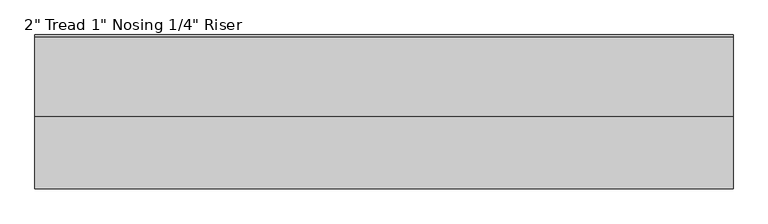
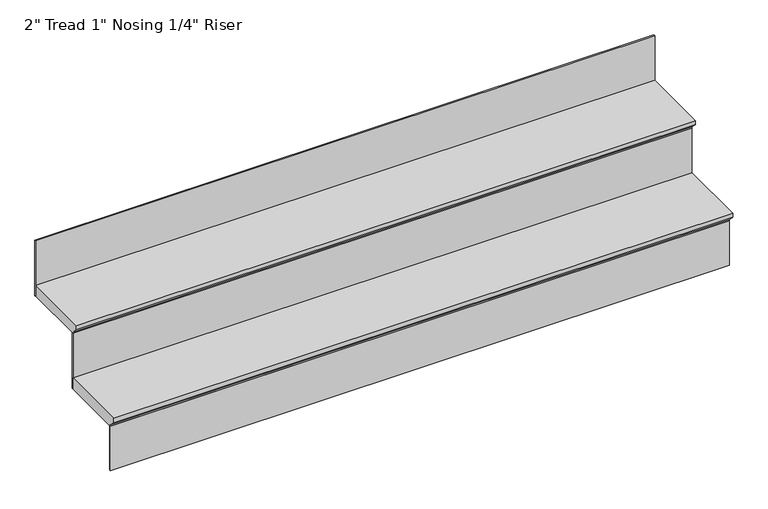
"""IFC4 building model written with IfcOpenShell, lengths in millimetres: stair flight geometry."""

from ifc_helpers import new_model, si_unit, frame, origin, place, context, project, spatial, polyline, outline, extrude, source, transform, mapped, element, save


def stair_flight_4a261924(model_context):
    return source(origin(), model_context, "Body", "SweptSolid", [
        extrude(outline(polyline([(409.2953049, -508.0), (714.0953049, -508.0), (714.0953049, -558.8), (434.6953049, -558.8), (434.6953049, -552.45), (409.2953049, -527.05), (409.2953049, -508.0)])), frame((-2797.3964374, 0.0, 0.0), z_axis=(1.0, 0.0, 0.0), x_axis=(0.0, 1.0, 0.0)), (0.0, 0.0, 1.0), 2678.1822327),
        extrude(outline(polyline([(-119.2142047, 441.0453049), (-119.2142047, 434.6953049), (-2797.3964374, 434.6953049), (-2797.3964374, 441.0453049), (-119.2142047, 441.0453049)])), frame((0.0, 0.0, -762.0), z_axis=(0.0, 0.0, 1.0), x_axis=(1.0, 0.0, 0.0)), (0.0, 0.0, 1.0), 203.2),
        extrude(outline(polyline([(-119.2142047, 720.4453049), (-119.2142047, 714.0953049), (-2797.3964374, 714.0953049), (-2797.3964374, 720.4453049), (-119.2142047, 720.4453049)])), frame((0.0, 0.0, -558.8), z_axis=(0.0, 0.0, 1.0), x_axis=(1.0, 0.0, 0.0)), (0.0, 0.0, 1.0), 254.0),
        extrude(outline(polyline([(-119.2142047, 999.8453049), (-119.2142047, 993.4953049), (-2797.3964374, 993.4953049), (-2797.3964374, 999.8453049), (-119.2142047, 999.8453049)])), frame((0.0, 0.0, -304.8), z_axis=(0.0, 0.0, 1.0), x_axis=(1.0, 0.0, 0.0)), (0.0, 0.0, 1.0), 254.0),
        extrude(outline(polyline([(688.6953049, -254.0), (993.4953049, -254.0), (993.4953049, -304.8), (714.0953049, -304.8), (714.0953049, -298.45), (688.6953049, -273.05), (688.6953049, -254.0)])), frame((-2797.3964374, 0.0, 0.0), z_axis=(1.0, 0.0, 0.0), x_axis=(0.0, 1.0, 0.0)), (0.0, 0.0, 1.0), 2678.1822327),
    ])


if __name__ == "__main__":
    model = new_model("IFC4")
    model_context = context("Model", 3, world=origin())
    ifc_project = project(units=[si_unit("LENGTHUNIT", "METRE", prefix="MILLI")], contexts=[model_context])
    site = spatial("IfcSite", under=ifc_project)
    building = spatial("IfcBuilding", under=site)
    placement = place(None, origin())
    stair_flight_shape = stair_flight_4a261924(model_context)
    element("IfcStairFlight", 1, ObjectType="2\" Tread 1\" Nosing 1/4\" Riser", at=placement, inside=building, context=model_context, shape_type="MappedRepresentation", body=[
        mapped(stair_flight_shape, transform((0.0, 0.0, 0.0), x_axis=(1.0, 0.0, 0.0), y_axis=(0.0, 1.0, 0.0), z_axis=(0.0, 0.0, 1.0))),
    ])
    save(model, "model.ifc")

# Revit data of these elements
# Element 1 (IfcStairFlight, "2\" Tread 1\" Nosing 1/4\" Riser")
#   Materials on its faces: "1 white"
# Materials
#   "1 white": class "Generic", colour RGB 244 245 241, transparency 0, Cost = 0
